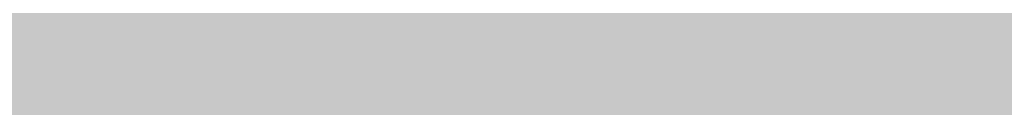
# Model space of a CAD drawing. Units: inches. Extents: x 2091 to 2899, y 967 to 2217.
# Tile 168 of 256: x 2203.14684 to 2203.151632, y 1152.24748 to 1152.2479. Entities that reach past the tile are written whole.
import ezdxf

# ---------------------------------------------------------------- set-up
doc = ezdxf.new("R2010")
doc.units = ezdxf.units.IN
doc.layers.add('A-WALL-PATT', color=141, linetype='Continuous', lineweight=13, true_color=0xadddf7)

msp = doc.modelspace()

# ---------------------------------------------------------------- hatches: boundary and pattern name
at = {"layer": 'A-WALL-PATT'}
h = msp.add_hatch(color=256, dxfattribs=at)
h.dxf.hatch_style = 1
h.paths.add_polyline_path([(2803.1436027, 2050.9190588), (2203.1436027, 2050.9190588), (2203.1436027, 1090.9190588), (2803.1436027, 1090.9190588)])
h.paths.add_polyline_path([(2635.7988501, 1147.5404649), (2674.5240524, 1147.5404649, 0.376086), (2678.5296653, 1152.8802017), (2678.5296653, 1159.5564734, 0.333335), (2674.524319, 1163.561846), (2674.524319, 1163.5618504), (2674.524319, 1192.9343904), (2635.8059707, 1192.9343904), (2597.0876225, 1192.9343904), (2597.0876225, 1163.561846, 0.333335), (2593.0822761, 1159.5564734), (2593.0822761, 1152.8802017, 0.376086), (2597.087889, 1147.5404649)], flags=0)
h.paths.add_polyline_path([(2436.0104329, 1278.2407784, 0.000483), (2435.9526433, 1278.215027, -0.001328), (2435.9356253, 1278.1116934, -0.001711), (2436.1164401, 1278.0407583, 0.002185)], flags=0)
h.paths.add_polyline_path([(2794.1436027, 1143.4190588), (2794.1436027, 1347.4190588), (2543.3701706, 1347.4190588), (2543.3701706, 1351.9190588), (2794.1436027, 1351.9190588), (2794.1436027, 1392.7135549), (2793.9473982, 1392.7135549), (2793.9473982, 1473.5368999), (2794.1436027, 1473.5368999), (2794.1436027, 1531.9190588), (2650.1436027, 1531.9190588), (2650.1436027, 1536.4190588), (2794.1436027, 1536.4190588), (2794.1436027, 1692.4190588), (2609.3756095, 1692.4190588), (2609.3756095, 1644.4190588), (2604.8756095, 1644.4190588), (2604.8756095, 1744.9190588), (2609.3756095, 1744.9190588), (2609.3756095, 1696.9190588), (2794.1436027, 1696.9190588), (2794.1436027, 1780.9190588), (2609.6436027, 1780.9190588), (2493.8756095, 1780.9190588), (2493.8756095, 1785.4190588), (2609.6436027, 1785.4190588), (2794.1436027, 1785.4190588), (2794.1436027, 1847.9388214), (2793.9512217, 1847.9388214), (2793.9512217, 1928.7621663), (2794.1436027, 1928.7621663), (2794.1436027, 1941.4190588), (2614.1436027, 1941.4190588), (2614.1436027, 1821.4190588), (2609.6436027, 1821.4190588), (2609.6436027, 1941.4190588), (2392.1436027, 1941.4190588), (2392.1436027, 1819.9190588), (2387.6436027, 1819.9190588), (2387.6436027, 1941.4190588), (2212.1436027, 1941.4190588), (2212.1436027, 1783.9190588), (2392.1436027, 1783.9190588), (2392.1436027, 1780.9190588), (2212.1436027, 1780.9190588), (2212.1436027, 1629.4190588), (2387.6436027, 1629.4190588), (2387.6436027, 1744.9190588), (2392.1436027, 1744.9190588), (2392.1436027, 1627.9190588), (2317.1436027, 1627.9190588), (2317.1436027, 1551.4190588), (2317.1436027, 1536.4190588), (2459.3835909, 1536.4190588), (2459.3835909, 1602.3964802), (2463.8835909, 1602.3964802), (2463.8835909, 1531.9190588), (2456.6436027, 1531.9190588), (2456.6436027, 1529.9190588), (2452.1436027, 1529.9190588), (2452.1436027, 1531.9190588), (2312.6436027, 1531.9190588), (2312.6436027, 1551.4190588), (2306.1436027, 1551.4190588), (2306.1436027, 1555.9190588), (2308.1436027, 1555.9190588), (2308.1436027, 1551.4190588), (2312.6436027, 1551.4190588), (2312.6436027, 1627.9190588), (2212.1436027, 1627.9190588), (2212.1436027, 1555.9190588), (2270.1436027, 1555.9190588), (2270.1436027, 1551.4190588), (2212.1436027, 1551.4190588), (2212.1436027, 1351.9190588), (2272.1436027, 1351.9190588), (2272.1436027, 1347.4190588), (2212.1436027, 1347.4190588), (2212.1436027, 1275.4190588), (2308.1436027, 1275.4190588), (2308.1436027, 1351.9190588), (2452.1436027, 1351.9190588), (2452.1436027, 1493.9190588), (2456.6436027, 1493.9190588), (2456.6436027, 1347.4190588), (2312.6436027, 1347.4190588), (2312.6436027, 1270.9190588), (2212.1436027, 1270.9190588), (2212.1436027, 1099.9190588), (2281.2375229, 1099.9190588), (2282.8710413, 1110.9138034), (2282.0083413, 1116.9966034), (2278.5577413, 1121.4204034), (2268.2056413, 1128.0562034), (2272.0876413, 1128.0562034), (2273.8129413, 1131.9270034), (2279.4203413, 1134.6919034), (2285.0278413, 1135.2449034), (2287.6158413, 1137.4568034), (2288.0471413, 1138.0098034), (2289.3411413, 1140.7747034), (2291.0665413, 1139.6687034), (2292.3605413, 1135.2449034), (2295.3798413, 1136.9038034), (2296.2425413, 1135.7979034), (2297.1052413, 1133.0330034), (2300.1246413, 1138.0098034), (2303.1439413, 1138.0098034), (2304.4379413, 1135.7979034), (2303.1439413, 1133.5860034), (2306.5946413, 1134.6919034), (2307.8887413, 1133.0330034), (2310.9080413, 1135.2449034), (2313.9274413, 1134.1389034), (2315.6268599, 1132.4271023), (2308.3200413, 1117.5496034), (2290.2038413, 1109.8079034), (2288.9098413, 1103.1721034), (2289.2723086, 1099.9190588), (2434.9182274, 1099.9190588), (2431.5932274, 1124.7880588), (2429.9302274, 1169.5530588), (2430.9271848, 1240.5196942), (2435.6589255, 1238.1861258), (2437.1352274, 1196.5540588), (2438.7982274, 1143.9730588), (2442.6782274, 1111.9980588), (2446.5582274, 1099.9190588), (2794.1436027, 1099.9190588), (2794.1436027, 1138.9190588), (2548.0324471, 1138.9190588), (2548.0324471, 1143.4190588), (2548.0324471, 1148.8190588), (2546.6684571, 1148.0315588), (2528.6856919, 1179.1786218, 0.256256), (2512.0324471, 1148.8190588), (2512.0324471, 1143.4190588), (2512.0324471, 1138.9190588), (2507.5324471, 1138.9190588), (2507.5324471, 1143.4190588), (2507.5324471, 1148.8190588, 0.256256), (2490.8792023, 1179.1786218), (2472.8964371, 1148.0315588), (2471.5324471, 1148.8190588), (2471.5324471, 1143.4190588), (2467.0324471, 1143.4190588), (2467.0324471, 1269.9457858, 0.039061), (2460.9099871, 1273.5800588), (2467.0324471, 1273.5800588), (2467.0324471, 1286.3253638, 0.014511), (2465.2161944, 1286.7619052), (2467.0324471, 1287.0525761), (2467.0324471, 1323.4190588), (2471.5324471, 1323.4190588), (2471.5324471, 1148.8190588), (2489.5324471, 1179.9959734), (2490.8964371, 1179.2084734), (2490.8792023, 1179.1786218, -0.256256), (2507.5324471, 1148.8190588), (2507.5324471, 1143.4190588), (2512.0324471, 1143.4190588), (2512.0324471, 1148.8190588, -0.256256), (2528.6856919, 1179.1786218), (2528.6684571, 1179.2084734), (2530.0324471, 1179.9959734), (2548.0324471, 1148.8190588), (2548.0324471, 1143.4190588)], flags=16)
h.paths.add_polyline_path([(2607.7685461, 1200.9450832), (2607.7685461, 1265.0306251), (2597.0876225, 1281.0520106), (2619.7845852, 1281.0520106), (2627.795278, 1337.1268598), (2635.7988501, 1337.1268598), (2643.8166634, 1337.1268598), (2651.8273562, 1281.0520106), (2674.524319, 1281.0520106), (2663.8433953, 1265.0306251), (2663.8433953, 1200.9450832), (2635.8059707, 1200.9450832)], flags=0)
edge = h.paths.add_edge_path(flags=0)
edge.add_ellipse((13303.8962153, 1272.9987247), major_axis=(-10595.3130399, 0.0000005), ratio=0.842303870086, start_angle=0.62823721906, end_angle=0.64655409989, ccw=False)
edge.add_ellipse((2711.7004495, 1156.8526781), major_axis=(2.2197691, 0), ratio=0.84230387, start_angle=111.5352435, end_angle=180.6282372, ccw=False)
edge.add_ellipse((13303.1562922, 1272.9987246), major_axis=(-10593.0263064, 0), ratio=0.842303869544, start_angle=0.52827147182, end_angle=0.64655409706, ccw=False)
edge.add_line((2710.7645961, 1175.3332951), (2710.1299858, 1175.3332951))
edge.add_ellipse((2710.1299858, 1176.5797752), major_axis=(1.4798461, 0), ratio=0.84230387, start_angle=180, end_angle=270, ccw=False)
edge.add_line((2708.6501397, 1176.5797752), (2708.6501397, 1200.7829144))
edge.add_ellipse((2710.1299858, 1200.7829144), major_axis=(1.4798461, 0), ratio=0.84230387, start_angle=90, end_angle=180, ccw=False)
edge.add_line((2710.1299858, 1202.0293944), (2710.4650752, 1202.0293944))
edge.add_ellipse((13303.1562922, 1272.9987246), major_axis=(-10593.0263064, 0), ratio=0.842303869544, start_angle=-0.09022908859, end_angle=0.38386677879, ccw=False)
edge.add_ellipse((2710.1299858, 1290.9270308), major_axis=(-1.4798461, 0), ratio=0.84230387, start_angle=0, end_angle=90, ccw=False)
edge.add_line((2708.6501397, 1290.9270308), (2708.6501397, 1315.13017))
edge.add_ellipse((2710.1299858, 1315.13017), major_axis=(-1.4798461, 0), ratio=0.84230387, start_angle=-90, end_angle=0, ccw=False)
edge.add_line((2710.1299858, 1316.3766501), (2710.7063141, 1316.3766501))
edge.add_ellipse((3238.4017202, 1296.2895655), major_axis=(528.2339998, 0), ratio=0.84230386954, start_angle=176.349572414, end_angle=177.820049686, ccw=False)
edge.add_ellipse((2775.0630432, 1071.4506962), major_axis=(313.3077613, 0), ratio=0.84230386954, start_angle=102.125965552, end_angle=103.780528989, ccw=False)
edge.add_ellipse((2775.0630432, 1078.3056979), major_axis=(-305.3028915, 0), ratio=0.84230386955, start_angle=-79.790461003, end_angle=-77.555372706, ccw=False)
edge.add_ellipse((2695.1417666, 1541.9753825), major_axis=(-250.9602162, 0), ratio=0.84230386954, start_angle=99.256566007, end_angle=102.554932644)
edge.add_line((2741.4103262, 1334.2142554), (2747.1325454, 1337.3784768))
edge.add_ellipse((2747.5386163, 1336.8574776), major_axis=(-0.739923, 0), ratio=0.84230387, start_angle=270, end_angle=307.9331305, ccw=False)
edge.add_ellipse((2747.5386163, 1336.8574776), major_axis=(-0.739923, 0), ratio=0.84230387, start_angle=232.0668695, end_angle=270, ccw=False)
edge.add_line((2747.9446872, 1337.3784768), (2753.6669064, 1334.2142554))
edge.add_ellipse((2799.935466, 1541.9753825), major_axis=(250.9602162, 0), ratio=0.84230386954, start_angle=257.445067356, end_angle=260.743433993)
edge.add_ellipse((2720.0141894, 1078.3056979), major_axis=(305.3028915, 0), ratio=0.84230386954, start_angle=77.555372707, end_angle=79.790461003, ccw=False)
edge.add_ellipse((2720.0141894, 1071.4506962), major_axis=(-313.3077613, 0), ratio=0.84230386954, start_angle=256.219471011, end_angle=257.874034448, ccw=False)
edge.add_ellipse((2256.6755124, 1296.2895655), major_axis=(-528.2339998, 0), ratio=0.84230386954, start_angle=182.179950314, end_angle=183.650427586, ccw=False)
edge.add_line((2784.3709184, 1316.3766501), (2784.9472468, 1316.3766501))
edge.add_ellipse((2784.9472468, 1315.13017), major_axis=(1.4798461, 0), ratio=0.84230387, start_angle=0, end_angle=90, ccw=False)
edge.add_line((2786.4270928, 1315.13017), (2786.4270928, 1290.9270308))
edge.add_ellipse((2784.9472468, 1290.9270308), major_axis=(1.4798461, 0), ratio=0.84230387, start_angle=270, end_angle=360, ccw=False)
edge.add_ellipse((-7808.0790596, 1272.9987246), major_axis=(10593.0263063, 0), ratio=0.842303869544, start_angle=-0.38386677879, end_angle=0.09022908859, ccw=False)
edge.add_line((2784.6121574, 1202.0293944), (2784.9472468, 1202.0293944))
edge.add_ellipse((2784.9472468, 1200.7829144), major_axis=(1.4798461, 0), ratio=0.84230387, start_angle=0, end_angle=90, ccw=False)
edge.add_line((2786.4270928, 1200.7829144), (2786.4270928, 1176.5797752))
edge.add_ellipse((2784.9472468, 1176.5797752), major_axis=(-1.4798461, 0), ratio=0.84230387, start_angle=90, end_angle=180, ccw=False)
edge.add_line((2784.9472468, 1175.3332951), (2784.3126365, 1175.3332951))
edge.add_ellipse((-7808.0790596, 1272.9987246), major_axis=(10593.0263063, 0), ratio=0.842303869544, start_angle=-0.61864319632, end_angle=-0.52827147182, ccw=False)
edge.add_ellipse((2783.3767831, 1156.8526781), major_axis=(-2.2197691, 0), ratio=0.84230387, start_angle=179.3717628, end_angle=248.4647566, ccw=False)
edge.add_ellipse((-7808.8189826, 1272.9987246), major_axis=(-10595.3130398, 0.0000036), ratio=0.842303865762, start_angle=179.3534459226, end_angle=179.37176280343, ccw=False)
edge.add_ellipse((2780.2973026, 1153.500793), major_axis=(-5.2464256, 0), ratio=0.84230387, start_angle=90, end_angle=179.3534459, ccw=False)
edge.add_line((2780.2973026, 1149.0817084), (2714.77993, 1149.0817084))
edge.add_ellipse((2714.77993, 1153.500793), major_axis=(5.2464256, 0), ratio=0.84230387, start_angle=180.6465541, end_angle=270, ccw=False)
edge = h.paths.add_edge_path(flags=0)
edge.add_line((2718.1873674, 1151.0078329), (2718.1873674, 1170.4723638))
edge.add_ellipse((2721.1470595, 1170.4723638), major_axis=(-2.9596921, 0), ratio=0.84230387, start_angle=-90, end_angle=0, ccw=False)
edge.add_line((2721.1470595, 1172.965324), (2773.9301731, 1172.965324))
edge.add_ellipse((2773.9301731, 1170.4723638), major_axis=(-2.9596921, 0), ratio=0.84230387, start_angle=180, end_angle=270, ccw=False)
edge.add_line((2776.8898652, 1170.4723638), (2776.8898652, 1151.0078329))
edge.add_line((2776.8898652, 1151.0078329), (2718.1873674, 1151.0078329))
edge = h.paths.add_edge_path(flags=0)
edge.add_line((2718.1873674, 1180.2341502), (2718.1873674, 1199.0578342))
edge.add_ellipse((2747.5386163, 1320.3986402), major_axis=(147.0179239, 0), ratio=0.84230386954, start_angle=256.40186531, end_angle=283.59813469)
edge.add_line((2776.8898652, 1199.0578342), (2776.8898652, 1180.2341502))
edge.add_ellipse((2747.5386163, 1301.5749562), major_axis=(147.0179239, 0), ratio=0.84230386954, start_angle=256.40186531, end_angle=283.59813469, ccw=False)
edge = h.paths.add_edge_path(flags=0)
edge.add_ellipse((13303.1562922, 1272.9987246), major_axis=(-10591.5464603, 0), ratio=0.842303869555, start_angle=0.05559431352, end_angle=0.37776419393, ccw=False)
edge.add_line((2711.6168595, 1262.7217103), (2715.6674076, 1249.4953957))
edge.add_ellipse((6413.8919626, 1241.691919), major_axis=(-3698.2361592, 0), ratio=0.842303869547, start_angle=-0.120897369, end_angle=0.3640763489)
edge.add_line((2715.7610383, 1218.1924547), (2711.9343065, 1203.167361))
edge = h.paths.add_edge_path(flags=0)
edge.add_line((2718.1873674, 1251.074566), (2716.0024854, 1267.4504351))
edge.add_ellipse((2742.1511746, 1202.1895399), major_axis=(81.7725845, 0), ratio=0.8423038695, start_angle=94.277420963, end_angle=111.834953797, ccw=False)
edge.add_line((2737.0097482, 1270.9306255), (2758.0674844, 1270.9306255))
edge.add_ellipse((2752.926058, 1202.1895399), major_axis=(81.7725845, 0), ratio=0.8423038695, start_angle=68.165046203, end_angle=85.722579037, ccw=False)
edge.add_line((2779.0747472, 1267.4504351), (2776.8898652, 1251.074566))
edge.add_ellipse((2750.3380588, 1187.8853558), major_axis=(79.5796641, 0), ratio=0.8423038695, start_angle=67.208085122, end_angle=85.129930403)
edge.add_line((2756.0346562, 1254.7436557), (2739.0425764, 1254.7436557))
edge.add_ellipse((2744.7391738, 1187.8853558), major_axis=(79.5796641, 0), ratio=0.8423038695, start_angle=94.870069597, end_angle=112.791914878)
edge = h.paths.add_edge_path(flags=0)
edge.add_line((2783.1429261, 1203.167361), (2779.3161943, 1218.1924547))
edge.add_ellipse((-918.81473, 1241.691919), major_axis=(3698.2361592, 0), ratio=0.842303869546, start_angle=-0.3640763489, end_angle=0.120897369)
edge.add_line((2779.409825, 1249.4953957), (2783.4603731, 1262.7217103))
edge.add_ellipse((-7808.0790596, 1272.9987246), major_axis=(-10591.5464603, 0), ratio=0.84230386954, start_angle=179.6222358061, end_angle=179.94440568651, ccw=False)
edge = h.paths.add_edge_path(flags=0)
edge.add_ellipse((2734.2008921, 1286.6904402), major_axis=(-0.3566086, 6.3400775), ratio=0.603833576, start_angle=89.00201428, end_angle=253.65740805, ccw=False)
edge.add_line((2730.3690013, 1286.5418057), (2730.3690013, 1301.3519803))
edge.add_line((2730.3690013, 1301.3519803), (2735.9133107, 1305.2148028))
edge.add_ellipse((2736.3849168, 1304.7345612), major_axis=(0.739923, 0), ratio=0.84230387, start_angle=90, end_angle=134.4802109, ccw=False)
edge.add_line((2736.3849168, 1305.3578013), (2738.0327829, 1305.3578013))
edge.add_line((2738.0327829, 1305.3578013), (2738.0327829, 1307.7079274))
edge.add_ellipse((2794.201642, 1307.7079274), major_axis=(56.168859, 0), ratio=0.8423038695, start_angle=150.5614304, end_angle=180, ccw=False)
edge.add_ellipse((2700.8755906, 1307.7079274), major_axis=(-56.168859, 0), ratio=0.8423038695, start_angle=180, end_angle=209.4385696, ccw=False)
edge.add_line((2757.0444497, 1307.7079274), (2757.0444497, 1305.3578013))
edge.add_line((2757.0444497, 1305.3578013), (2758.6923157, 1305.3578013))
edge.add_ellipse((2758.6923157, 1304.7345612), major_axis=(-0.739923, 0), ratio=0.84230387, start_angle=225.5197891, end_angle=270, ccw=False)
edge.add_line((2759.1639219, 1305.2148028), (2764.7082312, 1301.3519803))
edge.add_line((2764.7082312, 1301.3519803), (2764.7082312, 1286.5418057))
edge.add_ellipse((2760.8763405, 1286.6904402), major_axis=(0.3566086, 6.3400775), ratio=0.603833576, start_angle=106.34259195, end_angle=270.99798572, ccw=False)
edge.add_line((2757.0444497, 1285.7970896), (2757.0444497, 1307.7079274))
edge.add_ellipse((2700.8755906, 1307.7079274), major_axis=(-56.168859, 0), ratio=0.8423038695, start_angle=180, end_angle=209.4385696)
edge.add_ellipse((2794.201642, 1307.7079274), major_axis=(56.168859, 0), ratio=0.8423038695, start_angle=150.5614304, end_angle=180)
edge.add_line((2738.0327829, 1307.7079274), (2738.0327829, 1285.7970896))
h.paths.add_polyline_path([(2417.8122727, 1104.449704), (2413.4922727, 1102.529704), (2410.6122727, 1103.969704), (2409.1722727, 1106.369704), (2407.2522727, 1107.329704), (2406.2922727, 1109.729704), (2405.3322727, 1114.049704), (2405.3322727, 1117.889704), (2406.2922727, 1120.129704), (2407.2522727, 1119.809704), (2408.8483218, 1118.3276585), (2410.1739451, 1119.4241703), (2410.2112727, 1120.405704), (2411.0407305, 1121.4190541), (2410.6992727, 1119.858704), (2410.1739451, 1119.4241703), (2410.0884515, 1117.1761095), (2411.1328361, 1116.2063237), (2413.9722727, 1119.329704), (2416.8522727, 1120.769704), (2416.8697209, 1120.7987842), (2417.0350713, 1119.4051162), (2417.8962134, 1118.1433844), (2418.2922727, 1118.369704), (2419.5444467, 1120.0392692), (2419.3609153, 1118.387487), (2419.0321078, 1119.3561507), (2418.3989394, 1118.5119262), (2419.2522727, 1114.529704), (2418.7940909, 1107.1987949)], flags=0)
h.paths.add_polyline_path([(2508.8701706, 1347.4190588), (2508.3701706, 1347.4190588), (2508.3701706, 1351.9190588), (2508.8701706, 1351.9190588)], flags=0)
h.paths.add_polyline_path([(2473.3701706, 1347.4190588), (2472.3701706, 1347.4190588), (2467.8701706, 1347.4190588), (2467.8701706, 1455.4190588), (2472.3701706, 1455.4190588), (2472.3701706, 1352.4190588), (2473.3701706, 1352.4190588)], flags=0)
h.paths.add_polyline_path([(2352.106244, 1217.4461971), (2349.226244, 1218.8861971), (2347.786244, 1221.2861971), (2345.866244, 1222.2461971), (2344.906244, 1224.6461971), (2343.946244, 1228.9661971), (2343.946244, 1232.8061971), (2344.906244, 1235.0461971), (2345.866244, 1234.7261971), (2347.4622931, 1233.2441515), (2348.7879164, 1234.3406634), (2348.825244, 1235.3221971), (2349.6547018, 1236.3355471), (2349.313244, 1234.7751971), (2348.7879164, 1234.3406634), (2348.7024228, 1232.0926025), (2349.7468074, 1231.1228168), (2352.586244, 1234.2461971), (2355.466244, 1235.6861971), (2355.4836921, 1235.7152773), (2355.6490426, 1234.3216093), (2356.5101846, 1233.0598774), (2356.906244, 1233.2861971), (2358.1584179, 1234.9557623), (2357.9748866, 1233.3039801), (2357.6460791, 1234.2726438), (2357.0129107, 1233.4284193), (2357.866244, 1229.4461971), (2357.4080622, 1222.115288), (2356.426244, 1219.3661971)], flags=0)
h.paths.add_polyline_path([(2348.2967999, 1112.2244204), (2347.0137999, 1112.3104204), (2345.5297999, 1114.1274204), (2345.7317999, 1115.8584204), (2346.8117999, 1116.9824204), (2346.8117999, 1114.6464204), (2345.8667999, 1114.2144204), (2346.8797999, 1114.3004204)], flags=0)
h.paths.add_polyline_path([(2347.0137999, 1110.9264204), (2346.2717999, 1110.4934204), (2346.6097999, 1111.1864204)], flags=0)
h.paths.add_polyline_path([(2345.8667999, 1118.1944204), (2345.5297999, 1117.3294204), (2343.7077999, 1118.0214204), (2344.3827999, 1118.6264204)], flags=0)
h.paths.add_polyline_path([(2346.6767999, 1109.2824204), (2346.0697999, 1108.0714204), (2345.8667999, 1110.0614204)], flags=0)
h.paths.add_polyline_path([(2345.0567999, 1119.7514204), (2343.6397999, 1119.7514204), (2343.9777999, 1121.1354204)], flags=0)
h.paths.add_polyline_path([(2345.2597999, 1116.5504204), (2345.1247999, 1115.8584204), (2344.9217999, 1115.6854204), (2344.7197999, 1116.3774204)], flags=0)
h.paths.add_polyline_path([(2345.6647999, 1112.3104204), (2345.4617999, 1111.5324204), (2344.0447999, 1111.9644204), (2344.6517999, 1112.5704204)], flags=0)
h.paths.add_polyline_path([(2345.1917999, 1113.3494204), (2344.4497999, 1113.8684204), (2344.7197999, 1114.3874204)], flags=0)
h.paths.add_polyline_path([(2344.6517999, 1116.8094204), (2344.1797999, 1115.6854204), (2344.6517999, 1115.3394204), (2343.9097999, 1114.9064204), (2343.0327999, 1115.9444204), (2343.6397999, 1116.4634204)], flags=0)
h.paths.add_polyline_path([(2345.8667999, 1106.6864204), (2344.9897999, 1105.5624204), (2344.5167999, 1106.6004204)], flags=0)
h.paths.add_polyline_path([(2344.8547999, 1110.0614204), (2344.5167999, 1109.2824204), (2344.1127999, 1109.7154204)], flags=0)
h.paths.add_polyline_path([(2344.0447999, 1113.5224204), (2343.4377999, 1113.0894204), (2342.7627999, 1113.9544204)], flags=0)
h.paths.add_polyline_path([(2344.3147999, 1111.0124204), (2342.9647999, 1110.3204204), (2342.9647999, 1111.0994204)], flags=0)
h.paths.add_polyline_path([(2345.1247999, 1104.6974204), (2344.5847999, 1103.7454204), (2344.4497999, 1104.2644204)], flags=0)
h.paths.add_polyline_path([(2342.8297999, 1121.2224204), (2341.7497999, 1120.5304204), (2340.5357999, 1121.0494204), (2340.1307999, 1121.8284204), (2340.6707999, 1122.9524204), (2341.1427999, 1121.8284204), (2341.6147999, 1122.0014204)], flags=0)
h.paths.add_polyline_path([(2342.9647999, 1119.7514204), (2343.0327999, 1118.4534204), (2342.0877999, 1118.0214204), (2342.0197999, 1119.4914204)], flags=0)
h.paths.add_polyline_path([(2342.6947999, 1116.8964204), (2341.9527999, 1116.6364204), (2342.0197999, 1117.3294204)], flags=0)
h.paths.add_polyline_path([(2343.0327999, 1112.2244204), (2342.0197999, 1111.7914204), (2341.5477999, 1112.2244204), (2342.3577999, 1113.3494204)], flags=0)
h.paths.add_polyline_path([(2343.7747999, 1104.4374204), (2342.6277999, 1102.8804204), (2342.6947999, 1104.6104204), (2343.4377999, 1105.1294204)], flags=0)
h.paths.add_polyline_path([(2342.0197999, 1115.0794204), (2340.8057999, 1115.5124204), (2340.9407999, 1116.3774204)], flags=0)
h.paths.add_polyline_path([(2341.4807999, 1120.0974204), (2341.4807999, 1119.4054204), (2341.0757999, 1119.5784204), (2341.1427999, 1120.0974204)], flags=0)
h.paths.add_polyline_path([(2341.8177999, 1114.4734204), (2340.9407999, 1113.0894204), (2340.8057999, 1114.5604204)], flags=0)
h.paths.add_polyline_path([(2341.1427999, 1118.5404204), (2340.9407999, 1116.9824204), (2339.0507999, 1117.6754204), (2339.0507999, 1118.6264204)], flags=0)
h.paths.add_polyline_path([(2342.6947999, 1101.6684204), (2341.9527999, 1101.8414204), (2342.5597999, 1102.3614204)], flags=0)
h.paths.add_polyline_path([(2340.3327999, 1119.6654204), (2338.4437999, 1119.5784204), (2337.9037999, 1120.3574204), (2339.6577999, 1120.6164204)], flags=0)
h.paths.add_polyline_path([(2340.3327999, 1115.3394204), (2340.0627999, 1113.6954204), (2339.3877999, 1115.3394204)], flags=0)
h.paths.add_polyline_path([(2341.8177999, 1103.8314204), (2341.5477999, 1102.8804204), (2341.1427999, 1103.6584204)], flags=0)
h.paths.add_polyline_path([(2339.0507999, 1122.8664204), (2337.2957999, 1121.8284204), (2337.0937999, 1123.1254204), (2337.7687999, 1123.8184204)], flags=0)
h.paths.add_polyline_path([(2339.1177999, 1121.7414204), (2338.8477999, 1121.2224204), (2338.1737999, 1121.0494204), (2338.3757999, 1121.5684204)], flags=0)
h.paths.add_polyline_path([(2339.1857999, 1119.3194204), (2338.6457999, 1118.7134204), (2338.2407999, 1118.1074204), (2338.2407999, 1118.8864204)], flags=0)
h.paths.add_polyline_path([(2341.1427999, 1101.9284204), (2340.6027999, 1101.2364204), (2340.0627999, 1101.8414204), (2340.6027999, 1102.3614204)], flags=0)
h.paths.add_polyline_path([(2337.6337999, 1117.7614204), (2336.6207999, 1118.2804204), (2337.2957999, 1118.9724204)], flags=0)
h.paths.add_polyline_path([(2336.8237999, 1119.5784204), (2334.7987999, 1118.9724204), (2335.2037999, 1120.3574204), (2336.5537999, 1120.8764204)], flags=0)
h.paths.add_polyline_path([(2339.1177999, 1100.4574204), (2337.3637999, 1100.5434204), (2336.7557999, 1101.2364204)], flags=0)
h.paths.add_polyline_path([(2336.3507999, 1122.4334204), (2336.0137999, 1121.9144204), (2334.9337999, 1122.4334204), (2334.5287999, 1123.4714204), (2335.7437999, 1122.7794204)], flags=0)
h.paths.add_polyline_path([(2334.7317999, 1120.8764204), (2334.2587999, 1120.3574204), (2334.0567999, 1120.7894204), (2334.5967999, 1121.3084204)], flags=0)
h.paths.add_polyline_path([(2334.4617999, 1122.1744204), (2332.5717999, 1121.3084204), (2331.3567999, 1122.1744204), (2332.0997999, 1122.8664204)], flags=0)
h.paths.add_polyline_path([(2334.2587999, 1118.5404204), (2333.3817999, 1118.4534204), (2333.6517999, 1119.3194204)], flags=0)
h.paths.add_polyline_path([(2335.5417999, 1102.2744204), (2334.1917999, 1102.6204204), (2335.2717999, 1103.3124204)], flags=0)
h.paths.add_polyline_path([(2332.7067999, 1119.6654204), (2331.6947999, 1120.4434204), (2332.5047999, 1120.7894204)], flags=0)
h.paths.add_polyline_path([(2334.7317999, 1101.1494204), (2333.5167999, 1101.5824204), (2333.9887999, 1101.7554204)], flags=0)
h.paths.add_polyline_path([(2332.6397999, 1116.6364204), (2331.0867999, 1116.2904204), (2331.9647999, 1118.1944204)], flags=0)
h.paths.add_polyline_path([(2330.7497999, 1121.5684204), (2330.2767999, 1120.2704204), (2328.5227999, 1119.3194204), (2328.9947999, 1121.0494204)], flags=0)
h.paths.add_polyline_path([(2330.7497999, 1118.6264204), (2330.0077999, 1117.5024204), (2329.8727999, 1118.0214204)], flags=0)
h.paths.add_polyline_path([(2332.0997999, 1102.3614204), (2330.5467999, 1102.0144204), (2331.6947999, 1102.9664204)], flags=0)
h.paths.add_polyline_path([(2329.5347999, 1113.6084204), (2329.0627999, 1112.3104204), (2328.5897999, 1113.3494204)], flags=0)
h.paths.add_polyline_path([(2328.3877999, 1117.8484204), (2327.5097999, 1116.5504204), (2327.1727999, 1117.7614204)], flags=0)
h.paths.add_polyline_path([(2329.7377999, 1106.5134204), (2329.5347999, 1105.3024204), (2328.2527999, 1106.0814204)], flags=0)
h.paths.add_polyline_path([(2328.6577999, 1114.3874204), (2328.0497999, 1114.1274204), (2328.3197999, 1114.9064204)], flags=0)
h.paths.add_polyline_path([(2328.3197999, 1112.2244204), (2327.1057999, 1112.1374204), (2326.7007999, 1112.6564204)], flags=0)
h.paths.add_polyline_path([(2326.9027999, 1115.2524204), (2326.7007999, 1114.1274204), (2325.2157999, 1113.6084204), (2326.0927999, 1115.3394204)], flags=0)
h.paths.add_polyline_path([(2326.6327999, 1108.3304204), (2326.0927999, 1107.3794204), (2325.8907999, 1108.5034204), (2326.4977999, 1109.1094204)], flags=0)
h.paths.add_polyline_path([(2615.1436027, 1531.9190588), (2609.6436027, 1531.9190588), (2609.6436027, 1620.4190588), (2614.1436027, 1620.4190588), (2614.1436027, 1536.4190588), (2615.1436027, 1536.4190588)], flags=0)
h.paths.add_polyline_path([(2545.1436027, 1563.4190588), (2464.1436027, 1563.4190588), (2464.1436027, 1632.4190588), (2509.1436027, 1632.4190588), (2509.1436027, 1627.9190588), (2509.1436027, 1603.9190588), (2468.6436027, 1603.9190588), (2468.6436027, 1567.9190588), (2540.6436027, 1567.9190588), (2540.6436027, 1591.9190588), (2545.1436027, 1591.9190588)], flags=0)
h.paths.add_polyline_path([(2388.9690483, 1549.985735), (2357.4341811, 1549.985735), (2357.4341811, 1623.3607783), (2399.3627772, 1623.3607783), (2435.6894654, 1623.3607783), (2435.5925469, 1602.5592734), (2435.5925469, 1602.3964802), (2388.9690483, 1602.3964802)], flags=0)
h.paths.add_polyline_path([(2388.8806282, 1555.8091511), (2374.9044295, 1555.8091511), (2374.9044295, 1600.5715641), (2374.9044295, 1615.4576454), (2406.3508766, 1615.4576454), (2406.3508766, 1618.9394309), (2412.1742927, 1615.4576454), (2406.3508766, 1611.9758599), (2406.3508766, 1615.4576454), (2388.8806282, 1615.4576454)], flags=0)
h.paths.add_polyline_path([(2568.8756095, 1644.4190588), (2453.3756095, 1644.4190588), (2453.3756095, 1785.4190588), (2457.8756095, 1785.4190588), (2457.8756095, 1648.9190588), (2568.8756095, 1648.9190588)], flags=0)
h.paths.add_polyline_path([(2212.1436027, 1945.9190588), (2212.1436027, 2041.9190588), (2794.1436027, 2041.9190588), (2794.1436027, 1945.9190588)], flags=16)
h.paths.add_polyline_path([(2271.0827276, 1964.3172377), (2776.852968, 1964.3172377), (2776.852968, 2037.1696226), (2271.0827276, 2037.1696226)], flags=8)
h.paths.add_polyline_path([(2380.6492852, 1536.8241435), (2461.0408087, 1536.8241435), (2461.0408087, 1554.6525871), (2380.6492852, 1554.6525871)], flags=8)
h.paths.add_polyline_path([(2240.7557092, 1609.7254508), (2309.1858294, 1609.7254508), (2309.1858294, 1617.6982037), (2240.7557092, 1617.6982037)], flags=8)
h.paths.add_polyline_path([(2212.6772554, 1313.5041021), (2282.5915203, 1313.5041021), (2282.5915203, 1322.7452389), (2212.6772554, 1322.7452389)], flags=8)
h.paths.add_polyline_path([(2457.111976, 1114.778574), (2558.4815807, 1114.778574), (2558.4815807, 1142.2196823), (2457.111976, 1142.2196823)], flags=8)
h.paths.add_polyline_path([(2473.4423372, 1273.0100672), (2604.6412257, 1273.0100672), (2604.6412257, 1318.3469349), (2473.4423372, 1318.3469349)], flags=8)
h.paths.add_polyline_path([(2638.8763024, 1626.9774316), (2684.2503675, 1627.9767377), (2684.0384825, 1637.5974944), (2638.6644174, 1636.5981884)], flags=8)
h.paths.add_polyline_path([(2537.5905538, 1453.7934466), (2628.3895472, 1453.7934466), (2628.3895472, 1475.3448114), (2537.5905538, 1475.3448114)], flags=8)
h.paths.add_polyline_path([(2504.1376376, 1714.6323972), (2554.6471875, 1714.6323972), (2554.6471875, 1730.2377115), (2504.1376376, 1730.2377115)], flags=8)
h.paths.add_polyline_path([(2487.5011806, 1575.6518716), (2535.0971214, 1575.6518716), (2535.0971214, 1598.3776456), (2487.5011806, 1598.3776456)], flags=8)
h.paths.add_polyline_path([(2709.0994004, 1735.7102784), (2740.0166009, 1735.7102784), (2740.0166009, 1749.9376406), (2709.0994004, 1749.9376406)], flags=8)
h.paths.add_polyline_path([(2442.4384239, 1792.1716575), (2564.7288353, 1792.1716575), (2564.7288353, 1842.0001626), (2442.4384239, 1842.0001626)], flags=8)
h.paths.add_polyline_path([(2655.8158012, 1809.6440763), (2789.5201425, 1806.6937963), (2790.0849768, 1832.2916379), (2656.3806355, 1835.2419179)], flags=8)
h.paths.add_polyline_path([(2234.8426972, 1797.7201432), (2368.5928512, 1794.7688523), (2369.1607182, 1820.504132), (2235.4105642, 1823.4554229)], flags=8)
h.paths.add_polyline_path([(2245.1384659, 1644.0063348), (2398.4277329, 1640.6238997), (2398.9948417, 1666.3248199), (2245.7055747, 1669.7072549)], flags=8)
h.paths.add_polyline_path([(2306.1428474, 1431.1685186), (2413.7683138, 1428.7936873), (2414.3331481, 1454.3915289), (2306.7076817, 1456.7663602)], flags=8)
h.paths.add_polyline_path([(2306.834582, 1458.2331447), (2393.3804836, 1456.3234487), (2393.9328082, 1481.3543583), (2307.3869066, 1483.2640542)], flags=8)

doc.saveas('drawing.dxf')
